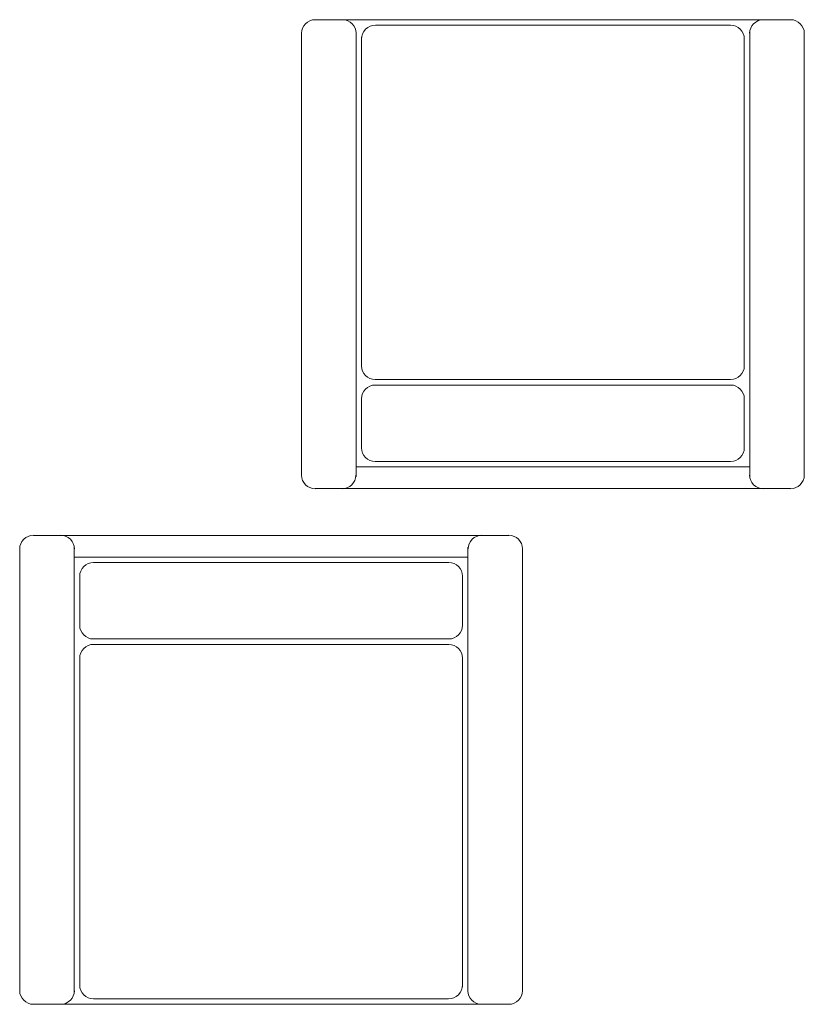
# Model space of a CAD drawing. Units: inches. Extents: x 205 to 1667, y -23 to 828.
# Tile 9 of 10: x 1050 to 1106, y 220 to 290. Entities that reach past the tile are written whole.
import ezdxf

# ---------------------------------------------------------------- set-up
doc = ezdxf.new("R2010")
doc.units = ezdxf.units.IN
doc.header["$MEASUREMENT"] = 0
doc.layers.add('A-FURN', color=8, linetype='Continuous', lineweight=18)

# ---------------------------------------------------------------- blocks, each defined once
blk = doc.blocks.new('CHAIR-LOUNGE')
for p, q in [((0.969, 33.327), (34.746, 33.327)), ((30.483, 32.939), (5.263, 32.939)), ((0, 0.968), (0, 32.358)), ((3.876, 0.832), (3.876, 32.457)), ((31.839, 32.479), (31.839, 0.87)), ((35.714, 32.358), (35.714, 0.968)), ((4.263, 8.719), (4.263, 31.939)), ((31.452, 31.97), (31.452, 8.719)), ((30.483, 7.75), (5.232, 7.75)), ((30.483, 7.363), (5.232, 7.363)), ((4.263, 2.906), (4.263, 6.394)), ((31.452, 6.394), (31.452, 2.906)), ((31.839, 1.55), (3.876, 1.55)), ((30.483, 1.937), (5.232, 1.937)), ((34.746, 0), (0.969, 0))]:
    blk.add_line(p, q)
for centre, radius, start, end in [((0.969, 32.358), 0.969, 90, 180), ((2.912, 32.358), 0.969, 0, 90), ((5.263, 31.939), 1, 90, 180), ((30.483, 31.97), 0.969, 0, 90), ((32.803, 32.358), 0.969, 90, 180), ((34.746, 32.358), 0.969, 0, 90), ((5.232, 31.97), 0.969, 169.61607, 180), ((5.232, 8.719), 0.969, 180, 270), ((30.483, 8.719), 0.969, 270, 0), ((5.232, 6.394), 0.969, 90, 180), ((30.483, 6.394), 0.969, 0, 90), ((5.232, 2.906), 0.969, 180, 270), ((30.483, 2.906), 0.969, 270, 0), ((0.969, 0.968), 0.969, 180, 270), ((2.898, 0.968), 0.969, 270, 0), ((32.803, 0.968), 0.969, 180, 270), ((34.746, 0.968), 0.969, 270, 0)]:
    blk.add_arc(centre, radius, start, end)

msp = doc.modelspace()

# ---------------------------------------------------------------- block references
at = {"layer": 'A-FURN'}
msp.add_blockref('CHAIR-LOUNGE', (1070.3259, 256.352), dxfattribs=at)
at = {"layer": 'A-FURN', "rotation": 180}
msp.add_blockref('CHAIR-LOUNGE', (1086.0289, 253.0353), dxfattribs=at)

doc.saveas('drawing.dxf')
